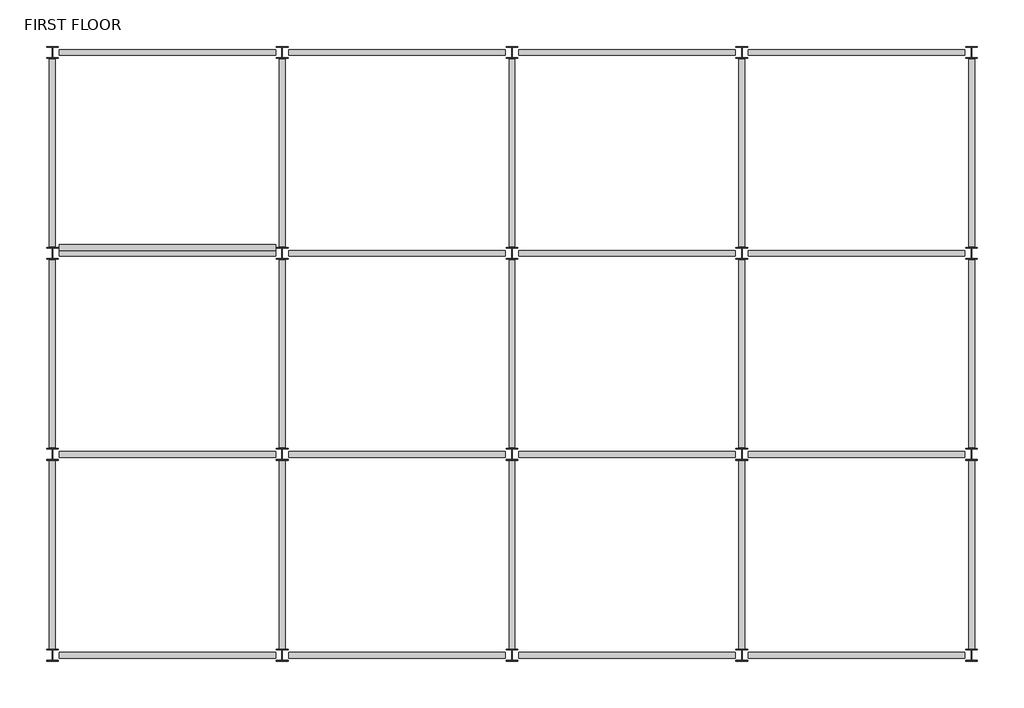
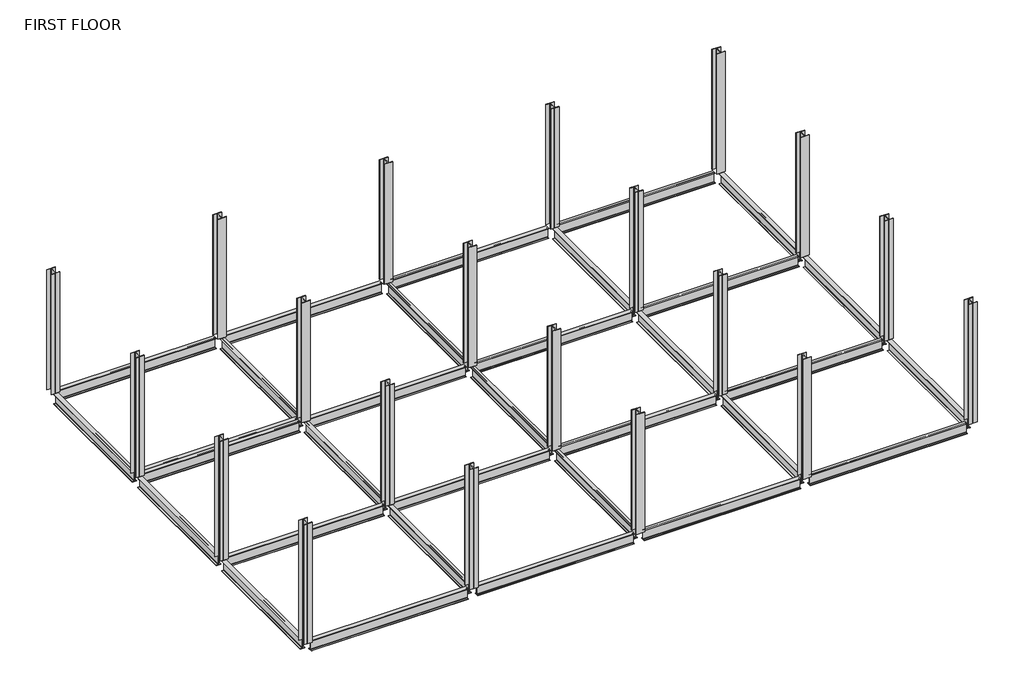
# One storey: 32 beams, 20 columns.
"""IFC4 building model written with IfcOpenShell, lengths in millimetres."""

from ifc_helpers import new_model, si_unit, origin, place, context, project, spatial, transform, mapped, element, save
from components import ub_universal_beams_ub254x102x28_022e5764, ub_universal_beams_ub254x102x28_3359efaf, ub_universal_beams_ub254x102x28_3001bc84, uc_universal_columns_column_uc203x203x52_fec190f4

model = new_model("IFC4")

# Units and contexts
model_context = context("Model", 3, world=origin())
ifc_project = project(units=[si_unit("LENGTHUNIT", "METRE", prefix="MILLI")], contexts=[model_context])

# Site, building, storey
site = spatial("IfcSite", under=ifc_project)
building = spatial("IfcBuilding", under=site)
storey = spatial("IfcBuildingStorey", under=building, Name="FIRST FLOOR", Elevation=3048.0)

# Beams
placement = place(None, origin())
ub_universal_beams_ub254x102x28_shape = ub_universal_beams_ub254x102x28_022e5764(model_context)
element("IfcBeam", 1, ObjectType="UB-Universal Beams : UB254x102x28", at=placement, inside=storey, context=model_context, shape_type="MappedRepresentation", body=[
    mapped(ub_universal_beams_ub254x102x28_shape, transform((-6871.2144105, 6458.2567898, 2917.8), x_axis=(1.0, 0.0, 0.0), y_axis=(0.0, 1.0, 0.0), z_axis=(0.0, 0.0, 1.0))),
])
ub_universal_beams_ub254x102x28_2_shape = ub_universal_beams_ub254x102x28_3359efaf(model_context)
element("IfcBeam", 2, ObjectType="UB-Universal Beams : UB254x102x28", at=placement, inside=storey, context=model_context, shape_type="MappedRepresentation", body=[
    mapped(ub_universal_beams_ub254x102x28_2_shape, transform((-8930.6620752, 1105.8028699, 2917.8), x_axis=(0.0, 1.0, 0.0), y_axis=(-1.0, 0.0, 0.0), z_axis=(0.0, 0.0, 1.0))),
])
element("IfcBeam", 3, ObjectType="UB-Universal Beams : UB254x102x28", at=placement, inside=storey, context=model_context, shape_type="MappedRepresentation", body=[
    mapped(ub_universal_beams_ub254x102x28_2_shape, transform((-8930.6620752, 4605.8028699, 2917.8), x_axis=(0.0, 1.0, 0.0), y_axis=(-1.0, 0.0, 0.0), z_axis=(0.0, 0.0, 1.0))),
])
element("IfcBeam", 4, ObjectType="UB-Universal Beams : UB254x102x28", at=placement, inside=storey, context=model_context, shape_type="MappedRepresentation", body=[
    mapped(ub_universal_beams_ub254x102x28_2_shape, transform((-8930.6620752, 8105.8028699, 2917.8), x_axis=(0.0, 1.0, 0.0), y_axis=(-1.0, 0.0, 0.0), z_axis=(0.0, 0.0, 1.0))),
])
element("IfcBeam", 5, ObjectType="UB-Universal Beams : UB254x102x28", at=placement, inside=storey, context=model_context, shape_type="MappedRepresentation", body=[
    mapped(ub_universal_beams_ub254x102x28_2_shape, transform((-4930.6620752, 1105.8028699, 2917.8), x_axis=(0.0, 1.0, 0.0), y_axis=(-1.0, 0.0, 0.0), z_axis=(0.0, 0.0, 1.0))),
])
element("IfcBeam", 6, ObjectType="UB-Universal Beams : UB254x102x28", at=placement, inside=storey, context=model_context, shape_type="MappedRepresentation", body=[
    mapped(ub_universal_beams_ub254x102x28_2_shape, transform((-4930.6620752, 4605.8028699, 2917.8), x_axis=(0.0, 1.0, 0.0), y_axis=(-1.0, 0.0, 0.0), z_axis=(0.0, 0.0, 1.0))),
])
element("IfcBeam", 7, ObjectType="UB-Universal Beams : UB254x102x28", at=placement, inside=storey, context=model_context, shape_type="MappedRepresentation", body=[
    mapped(ub_universal_beams_ub254x102x28_2_shape, transform((-4930.6620752, 8105.8028699, 2917.8), x_axis=(0.0, 1.0, 0.0), y_axis=(-1.0, 0.0, 0.0), z_axis=(0.0, 0.0, 1.0))),
])
element("IfcBeam", 8, ObjectType="UB-Universal Beams : UB254x102x28", at=placement, inside=storey, context=model_context, shape_type="MappedRepresentation", body=[
    mapped(ub_universal_beams_ub254x102x28_2_shape, transform((-930.6620752, 1105.8028699, 2917.8), x_axis=(0.0, 1.0, 0.0), y_axis=(-1.0, 0.0, 0.0), z_axis=(0.0, 0.0, 1.0))),
])
element("IfcBeam", 9, ObjectType="UB-Universal Beams : UB254x102x28", at=placement, inside=storey, context=model_context, shape_type="MappedRepresentation", body=[
    mapped(ub_universal_beams_ub254x102x28_2_shape, transform((-930.6620752, 4605.8028699, 2917.8), x_axis=(0.0, 1.0, 0.0), y_axis=(-1.0, 0.0, 0.0), z_axis=(0.0, 0.0, 1.0))),
])
element("IfcBeam", 10, ObjectType="UB-Universal Beams : UB254x102x28", at=placement, inside=storey, context=model_context, shape_type="MappedRepresentation", body=[
    mapped(ub_universal_beams_ub254x102x28_2_shape, transform((-930.6620752, 8105.8028699, 2917.8), x_axis=(0.0, 1.0, 0.0), y_axis=(-1.0, 0.0, 0.0), z_axis=(0.0, 0.0, 1.0))),
])
element("IfcBeam", 11, ObjectType="UB-Universal Beams : UB254x102x28", at=placement, inside=storey, context=model_context, shape_type="MappedRepresentation", body=[
    mapped(ub_universal_beams_ub254x102x28_2_shape, transform((3069.3379248, 1105.8028699, 2917.8), x_axis=(0.0, 1.0, 0.0), y_axis=(-1.0, 0.0, 0.0), z_axis=(0.0, 0.0, 1.0))),
])
element("IfcBeam", 12, ObjectType="UB-Universal Beams : UB254x102x28", at=placement, inside=storey, context=model_context, shape_type="MappedRepresentation", body=[
    mapped(ub_universal_beams_ub254x102x28_2_shape, transform((3069.3379248, 4605.8028699, 2917.8), x_axis=(0.0, 1.0, 0.0), y_axis=(-1.0, 0.0, 0.0), z_axis=(0.0, 0.0, 1.0))),
])
element("IfcBeam", 13, ObjectType="UB-Universal Beams : UB254x102x28", at=placement, inside=storey, context=model_context, shape_type="MappedRepresentation", body=[
    mapped(ub_universal_beams_ub254x102x28_2_shape, transform((3069.3379248, 8105.8028699, 2917.8), x_axis=(0.0, 1.0, 0.0), y_axis=(-1.0, 0.0, 0.0), z_axis=(0.0, 0.0, 1.0))),
])
element("IfcBeam", 14, ObjectType="UB-Universal Beams : UB254x102x28", at=placement, inside=storey, context=model_context, shape_type="MappedRepresentation", body=[
    mapped(ub_universal_beams_ub254x102x28_2_shape, transform((7069.3379248, 1105.8028699, 2917.8), x_axis=(0.0, 1.0, 0.0), y_axis=(-1.0, 0.0, 0.0), z_axis=(0.0, 0.0, 1.0))),
])
element("IfcBeam", 15, ObjectType="UB-Universal Beams : UB254x102x28", at=placement, inside=storey, context=model_context, shape_type="MappedRepresentation", body=[
    mapped(ub_universal_beams_ub254x102x28_2_shape, transform((7069.3379248, 4605.8028699, 2917.8), x_axis=(0.0, 1.0, 0.0), y_axis=(-1.0, 0.0, 0.0), z_axis=(0.0, 0.0, 1.0))),
])
element("IfcBeam", 16, ObjectType="UB-Universal Beams : UB254x102x28", at=placement, inside=storey, context=model_context, shape_type="MappedRepresentation", body=[
    mapped(ub_universal_beams_ub254x102x28_2_shape, transform((7069.3379248, 8105.8028699, 2917.8), x_axis=(0.0, 1.0, 0.0), y_axis=(-1.0, 0.0, 0.0), z_axis=(0.0, 0.0, 1.0))),
])
ub_universal_beams_ub254x102x28_3_shape = ub_universal_beams_ub254x102x28_3001bc84(model_context)
element("IfcBeam", 17, ObjectType="UB-Universal Beams : UB254x102x28", at=placement, inside=storey, context=model_context, shape_type="MappedRepresentation", body=[
    mapped(ub_universal_beams_ub254x102x28_3_shape, transform((-6930.6620752, 9855.8028699, 2917.8), x_axis=(1.0, 0.0, 0.0), y_axis=(0.0, 1.0, 0.0), z_axis=(0.0, 0.0, 1.0))),
])
element("IfcBeam", 18, ObjectType="UB-Universal Beams : UB254x102x28", at=placement, inside=storey, context=model_context, shape_type="MappedRepresentation", body=[
    mapped(ub_universal_beams_ub254x102x28_3_shape, transform((-2930.6620752, 9855.8028699, 2917.8), x_axis=(1.0, 0.0, 0.0), y_axis=(0.0, 1.0, 0.0), z_axis=(0.0, 0.0, 1.0))),
])
element("IfcBeam", 19, ObjectType="UB-Universal Beams : UB254x102x28", at=placement, inside=storey, context=model_context, shape_type="MappedRepresentation", body=[
    mapped(ub_universal_beams_ub254x102x28_3_shape, transform((1069.3379248, 9855.8028699, 2917.8), x_axis=(1.0, 0.0, 0.0), y_axis=(0.0, 1.0, 0.0), z_axis=(0.0, 0.0, 1.0))),
])
element("IfcBeam", 20, ObjectType="UB-Universal Beams : UB254x102x28", at=placement, inside=storey, context=model_context, shape_type="MappedRepresentation", body=[
    mapped(ub_universal_beams_ub254x102x28_3_shape, transform((5069.3379248, 9855.8028699, 2917.8), x_axis=(1.0, 0.0, 0.0), y_axis=(0.0, 1.0, 0.0), z_axis=(0.0, 0.0, 1.0))),
])
element("IfcBeam", 21, ObjectType="UB-Universal Beams : UB254x102x28", at=placement, inside=storey, context=model_context, shape_type="MappedRepresentation", body=[
    mapped(ub_universal_beams_ub254x102x28_3_shape, transform((-6930.6620752, 6355.8028699, 2917.8), x_axis=(1.0, 0.0, 0.0), y_axis=(0.0, 1.0, 0.0), z_axis=(0.0, 0.0, 1.0))),
])
element("IfcBeam", 22, ObjectType="UB-Universal Beams : UB254x102x28", at=placement, inside=storey, context=model_context, shape_type="MappedRepresentation", body=[
    mapped(ub_universal_beams_ub254x102x28_3_shape, transform((-2930.6620752, 6355.8028699, 2917.8), x_axis=(1.0, 0.0, 0.0), y_axis=(0.0, 1.0, 0.0), z_axis=(0.0, 0.0, 1.0))),
])
element("IfcBeam", 23, ObjectType="UB-Universal Beams : UB254x102x28", at=placement, inside=storey, context=model_context, shape_type="MappedRepresentation", body=[
    mapped(ub_universal_beams_ub254x102x28_3_shape, transform((1069.3379248, 6355.8028699, 2917.8), x_axis=(1.0, 0.0, 0.0), y_axis=(0.0, 1.0, 0.0), z_axis=(0.0, 0.0, 1.0))),
])
element("IfcBeam", 24, ObjectType="UB-Universal Beams : UB254x102x28", at=placement, inside=storey, context=model_context, shape_type="MappedRepresentation", body=[
    mapped(ub_universal_beams_ub254x102x28_3_shape, transform((5069.3379248, 6355.8028699, 2917.8), x_axis=(1.0, 0.0, 0.0), y_axis=(0.0, 1.0, 0.0), z_axis=(0.0, 0.0, 1.0))),
])
element("IfcBeam", 25, ObjectType="UB-Universal Beams : UB254x102x28", at=placement, inside=storey, context=model_context, shape_type="MappedRepresentation", body=[
    mapped(ub_universal_beams_ub254x102x28_3_shape, transform((-6930.6620752, 2855.8028699, 2917.8), x_axis=(1.0, 0.0, 0.0), y_axis=(0.0, 1.0, 0.0), z_axis=(0.0, 0.0, 1.0))),
])
element("IfcBeam", 26, ObjectType="UB-Universal Beams : UB254x102x28", at=placement, inside=storey, context=model_context, shape_type="MappedRepresentation", body=[
    mapped(ub_universal_beams_ub254x102x28_3_shape, transform((-2930.6620752, 2855.8028699, 2917.8), x_axis=(1.0, 0.0, 0.0), y_axis=(0.0, 1.0, 0.0), z_axis=(0.0, 0.0, 1.0))),
])
element("IfcBeam", 27, ObjectType="UB-Universal Beams : UB254x102x28", at=placement, inside=storey, context=model_context, shape_type="MappedRepresentation", body=[
    mapped(ub_universal_beams_ub254x102x28_3_shape, transform((1069.3379248, 2855.8028699, 2917.8), x_axis=(1.0, 0.0, 0.0), y_axis=(0.0, 1.0, 0.0), z_axis=(0.0, 0.0, 1.0))),
])
element("IfcBeam", 28, ObjectType="UB-Universal Beams : UB254x102x28", at=placement, inside=storey, context=model_context, shape_type="MappedRepresentation", body=[
    mapped(ub_universal_beams_ub254x102x28_3_shape, transform((5069.3379248, 2855.8028699, 2917.8), x_axis=(1.0, 0.0, 0.0), y_axis=(0.0, 1.0, 0.0), z_axis=(0.0, 0.0, 1.0))),
])
element("IfcBeam", 29, ObjectType="UB-Universal Beams : UB254x102x28", at=placement, inside=storey, context=model_context, shape_type="MappedRepresentation", body=[
    mapped(ub_universal_beams_ub254x102x28_3_shape, transform((-6930.6620752, -644.1971301, 2917.8), x_axis=(1.0, 0.0, 0.0), y_axis=(0.0, 1.0, 0.0), z_axis=(0.0, 0.0, 1.0))),
])
element("IfcBeam", 30, ObjectType="UB-Universal Beams : UB254x102x28", at=placement, inside=storey, context=model_context, shape_type="MappedRepresentation", body=[
    mapped(ub_universal_beams_ub254x102x28_3_shape, transform((-2930.6620752, -644.1971301, 2917.8), x_axis=(1.0, 0.0, 0.0), y_axis=(0.0, 1.0, 0.0), z_axis=(0.0, 0.0, 1.0))),
])
element("IfcBeam", 31, ObjectType="UB-Universal Beams : UB254x102x28", at=placement, inside=storey, context=model_context, shape_type="MappedRepresentation", body=[
    mapped(ub_universal_beams_ub254x102x28_3_shape, transform((1069.3379248, -644.1971301, 2917.8), x_axis=(1.0, 0.0, 0.0), y_axis=(0.0, 1.0, 0.0), z_axis=(0.0, 0.0, 1.0))),
])
element("IfcBeam", 32, ObjectType="UB-Universal Beams : UB254x102x28", at=placement, inside=storey, context=model_context, shape_type="MappedRepresentation", body=[
    mapped(ub_universal_beams_ub254x102x28_3_shape, transform((5069.3379248, -644.1971301, 2917.8), x_axis=(1.0, 0.0, 0.0), y_axis=(0.0, 1.0, 0.0), z_axis=(0.0, 0.0, 1.0))),
])

# Columns
uc_universal_columns_column_uc203x203x52_shape = uc_universal_columns_column_uc203x203x52_fec190f4(model_context)
element("IfcColumn", 33, ObjectType="UC-Universal Columns-Column : UC203x203x52", at=placement, inside=storey, context=model_context, shape_type="MappedRepresentation", body=[
    mapped(uc_universal_columns_column_uc203x203x52_shape, transform((-8930.6620752, 9855.8028699, 0.0), x_axis=(1.0, 0.0, 0.0), y_axis=(0.0, 1.0, 0.0), z_axis=(0.0, 0.0, 1.0))),
])
element("IfcColumn", 34, ObjectType="UC-Universal Columns-Column : UC203x203x52", at=placement, inside=storey, context=model_context, shape_type="MappedRepresentation", body=[
    mapped(uc_universal_columns_column_uc203x203x52_shape, transform((-8930.6620752, 6355.8028699, 0.0), x_axis=(1.0, 0.0, 0.0), y_axis=(0.0, 1.0, 0.0), z_axis=(0.0, 0.0, 1.0))),
])
element("IfcColumn", 35, ObjectType="UC-Universal Columns-Column : UC203x203x52", at=placement, inside=storey, context=model_context, shape_type="MappedRepresentation", body=[
    mapped(uc_universal_columns_column_uc203x203x52_shape, transform((-8930.6620752, 2855.8028699, 0.0), x_axis=(1.0, 0.0, 0.0), y_axis=(0.0, 1.0, 0.0), z_axis=(0.0, 0.0, 1.0))),
])
element("IfcColumn", 36, ObjectType="UC-Universal Columns-Column : UC203x203x52", at=placement, inside=storey, context=model_context, shape_type="MappedRepresentation", body=[
    mapped(uc_universal_columns_column_uc203x203x52_shape, transform((-8930.6620752, -644.1971301, 0.0), x_axis=(1.0, 0.0, 0.0), y_axis=(0.0, 1.0, 0.0), z_axis=(0.0, 0.0, 1.0))),
])
element("IfcColumn", 37, ObjectType="UC-Universal Columns-Column : UC203x203x52", at=placement, inside=storey, context=model_context, shape_type="MappedRepresentation", body=[
    mapped(uc_universal_columns_column_uc203x203x52_shape, transform((-4930.6620752, 9855.8028699, 0.0), x_axis=(1.0, 0.0, 0.0), y_axis=(0.0, 1.0, 0.0), z_axis=(0.0, 0.0, 1.0))),
])
element("IfcColumn", 38, ObjectType="UC-Universal Columns-Column : UC203x203x52", at=placement, inside=storey, context=model_context, shape_type="MappedRepresentation", body=[
    mapped(uc_universal_columns_column_uc203x203x52_shape, transform((-4930.6620752, 6355.8028699, 0.0), x_axis=(1.0, 0.0, 0.0), y_axis=(0.0, 1.0, 0.0), z_axis=(0.0, 0.0, 1.0))),
])
element("IfcColumn", 39, ObjectType="UC-Universal Columns-Column : UC203x203x52", at=placement, inside=storey, context=model_context, shape_type="MappedRepresentation", body=[
    mapped(uc_universal_columns_column_uc203x203x52_shape, transform((-4930.6620752, 2855.8028699, 0.0), x_axis=(1.0, 0.0, 0.0), y_axis=(0.0, 1.0, 0.0), z_axis=(0.0, 0.0, 1.0))),
])
element("IfcColumn", 40, ObjectType="UC-Universal Columns-Column : UC203x203x52", at=placement, inside=storey, context=model_context, shape_type="MappedRepresentation", body=[
    mapped(uc_universal_columns_column_uc203x203x52_shape, transform((-4930.6620752, -644.1971301, 0.0), x_axis=(1.0, 0.0, 0.0), y_axis=(0.0, 1.0, 0.0), z_axis=(0.0, 0.0, 1.0))),
])
element("IfcColumn", 41, ObjectType="UC-Universal Columns-Column : UC203x203x52", at=placement, inside=storey, context=model_context, shape_type="MappedRepresentation", body=[
    mapped(uc_universal_columns_column_uc203x203x52_shape, transform((-930.6620752, 9855.8028699, 0.0), x_axis=(1.0, 0.0, 0.0), y_axis=(0.0, 1.0, 0.0), z_axis=(0.0, 0.0, 1.0))),
])
element("IfcColumn", 42, ObjectType="UC-Universal Columns-Column : UC203x203x52", at=placement, inside=storey, context=model_context, shape_type="MappedRepresentation", body=[
    mapped(uc_universal_columns_column_uc203x203x52_shape, transform((-930.6620752, 6355.8028699, 0.0), x_axis=(1.0, 0.0, 0.0), y_axis=(0.0, 1.0, 0.0), z_axis=(0.0, 0.0, 1.0))),
])
element("IfcColumn", 43, ObjectType="UC-Universal Columns-Column : UC203x203x52", at=placement, inside=storey, context=model_context, shape_type="MappedRepresentation", body=[
    mapped(uc_universal_columns_column_uc203x203x52_shape, transform((-930.6620752, 2855.8028699, 0.0), x_axis=(1.0, 0.0, 0.0), y_axis=(0.0, 1.0, 0.0), z_axis=(0.0, 0.0, 1.0))),
])
element("IfcColumn", 44, ObjectType="UC-Universal Columns-Column : UC203x203x52", at=placement, inside=storey, context=model_context, shape_type="MappedRepresentation", body=[
    mapped(uc_universal_columns_column_uc203x203x52_shape, transform((-930.6620752, -644.1971301, 0.0), x_axis=(1.0, 0.0, 0.0), y_axis=(0.0, 1.0, 0.0), z_axis=(0.0, 0.0, 1.0))),
])
element("IfcColumn", 45, ObjectType="UC-Universal Columns-Column : UC203x203x52", at=placement, inside=storey, context=model_context, shape_type="MappedRepresentation", body=[
    mapped(uc_universal_columns_column_uc203x203x52_shape, transform((3069.3379248, 9855.8028699, 0.0), x_axis=(1.0, 0.0, 0.0), y_axis=(0.0, 1.0, 0.0), z_axis=(0.0, 0.0, 1.0))),
])
element("IfcColumn", 46, ObjectType="UC-Universal Columns-Column : UC203x203x52", at=placement, inside=storey, context=model_context, shape_type="MappedRepresentation", body=[
    mapped(uc_universal_columns_column_uc203x203x52_shape, transform((3069.3379248, 6355.8028699, 0.0), x_axis=(1.0, 0.0, 0.0), y_axis=(0.0, 1.0, 0.0), z_axis=(0.0, 0.0, 1.0))),
])
element("IfcColumn", 47, ObjectType="UC-Universal Columns-Column : UC203x203x52", at=placement, inside=storey, context=model_context, shape_type="MappedRepresentation", body=[
    mapped(uc_universal_columns_column_uc203x203x52_shape, transform((3069.3379248, 2855.8028699, 0.0), x_axis=(1.0, 0.0, 0.0), y_axis=(0.0, 1.0, 0.0), z_axis=(0.0, 0.0, 1.0))),
])
element("IfcColumn", 48, ObjectType="UC-Universal Columns-Column : UC203x203x52", at=placement, inside=storey, context=model_context, shape_type="MappedRepresentation", body=[
    mapped(uc_universal_columns_column_uc203x203x52_shape, transform((3069.3379248, -644.1971301, 0.0), x_axis=(1.0, 0.0, 0.0), y_axis=(0.0, 1.0, 0.0), z_axis=(0.0, 0.0, 1.0))),
])
element("IfcColumn", 49, ObjectType="UC-Universal Columns-Column : UC203x203x52", at=placement, inside=storey, context=model_context, shape_type="MappedRepresentation", body=[
    mapped(uc_universal_columns_column_uc203x203x52_shape, transform((7069.3379248, 9855.8028699, 0.0), x_axis=(1.0, 0.0, 0.0), y_axis=(0.0, 1.0, 0.0), z_axis=(0.0, 0.0, 1.0))),
])
element("IfcColumn", 50, ObjectType="UC-Universal Columns-Column : UC203x203x52", at=placement, inside=storey, context=model_context, shape_type="MappedRepresentation", body=[
    mapped(uc_universal_columns_column_uc203x203x52_shape, transform((7069.3379248, 6355.8028699, 0.0), x_axis=(1.0, 0.0, 0.0), y_axis=(0.0, 1.0, 0.0), z_axis=(0.0, 0.0, 1.0))),
])
element("IfcColumn", 51, ObjectType="UC-Universal Columns-Column : UC203x203x52", at=placement, inside=storey, context=model_context, shape_type="MappedRepresentation", body=[
    mapped(uc_universal_columns_column_uc203x203x52_shape, transform((7069.3379248, 2855.8028699, 0.0), x_axis=(1.0, 0.0, 0.0), y_axis=(0.0, 1.0, 0.0), z_axis=(0.0, 0.0, 1.0))),
])
element("IfcColumn", 52, ObjectType="UC-Universal Columns-Column : UC203x203x52", at=placement, inside=storey, context=model_context, shape_type="MappedRepresentation", body=[
    mapped(uc_universal_columns_column_uc203x203x52_shape, transform((7069.3379248, -644.1971301, 0.0), x_axis=(1.0, 0.0, 0.0), y_axis=(0.0, 1.0, 0.0), z_axis=(0.0, 0.0, 1.0))),
])

save(model, "model.ifc")

# Revit data of these elements
# Type "UB-Universal Beams : UB254x102x28"
#   Section Name Key = "UB254X102X28"
#   Width = 10.22 cm
#   Web Thickness = 0.63 cm
#   Web Fillet = 0.76 cm
#   Warping Constant = 28000.0 cm⁶
#   Torsional Moment of Inertia = 9.57 cm⁴
#   Section Area = 36.1 cm²
#   Plastic Modulus weak axis = 54.8 cm³
#   Plastic Modulus strong axis = 353.0 cm³
#   Nominal Weight = 28.2999 kgf/m
#   Moment of Inertia weak axis = 179.00 cm⁴
#   Moment of Inertia strong axis = 4005.00 cm⁴
#   Height = 26.04 cm
#   Flange Thickness = 1.0 cm
#   Elastic Modulus weak axis = 34.9 cm³
#   Elastic Modulus strong axis = 308.0 cm³
#   Centroid Vertical = 13.02 cm
#   Centroid Horizontal = 5.11 cm
#   Bolt Spacing = 5.4 cm
#   Length [instance default] = 4' - 11.05512"
#   Structural Material [instance default] = Metal - Steel 43-275
#   Type Comments = ""
#   Assembly Code = ""
# Type "UC-Universal Columns-Column : UC203x203x52"
#   Section Name Key = "UC203x203x52"
#   Width = 20.43 cm
#   Web Thickness = 0.79 cm
#   Web Fillet = 1.02 cm
#   Warping Constant = 167000.0 cm⁶
#   Torsional Moment of Inertia = 31.80 cm⁴
#   Section Area = 66.0 cm²
#   Plastic Modulus weak axis = 264.0 cm³
#   Plastic Modulus strong axis = 567.0 cm³
#   Nominal Weight = 51.9998 kgf/m
#   Moment of Inertia weak axis = 1778.00 cm⁴
#   Moment of Inertia strong axis = 5259.00 cm⁴
#   Height = 20.62 cm
#   Flange Thickness = 1.25 cm
#   Elastic Modulus weak axis = 174.0 cm³
#   Elastic Modulus strong axis = 510.0 cm³
#   Centroid Vertical = 10.31 cm
#   Centroid Horizontal = 10.215 cm
#   Bolt Spacing = 14.0 cm
#   Structural Material [instance default] = Metal - Steel 43-275
#   Type Comments = ""
#   Assembly Code = ""
# Elements 1, 2, 3, 4, 5, 6, 7, 8, 9, 10, 11, 12, 13, 14, 15, 16, 17, 18, 19, 20, 21, 22, 23, 24, 25, 26, 27, 28, 29, 30, 31, 32 (IfcBeam, "UB-Universal Beams : UB254x102x28")
#   Structural Material = Metal - Steel 43-275
#   Phase Created = New Construction
#   Materials on its faces: "Metal - Steel 43-275"
# Elements 33, 34, 35, 36, 37, 38, 39, 40, 41, 42, 43, 44, 45, 46, 47, 48, 49, 50, 51, 52 (IfcColumn, "UC-Universal Columns-Column : UC203x203x52")
#   Structural Material = Metal - Steel 43-275
#   Phase Created = New Construction
#   Materials on its faces: "Metal - Steel 43-275"
# Materials
#   "Metal - Steel 43-275": class "Metal", colour RGB 247 247 247, transparency 0, Cost = 0
